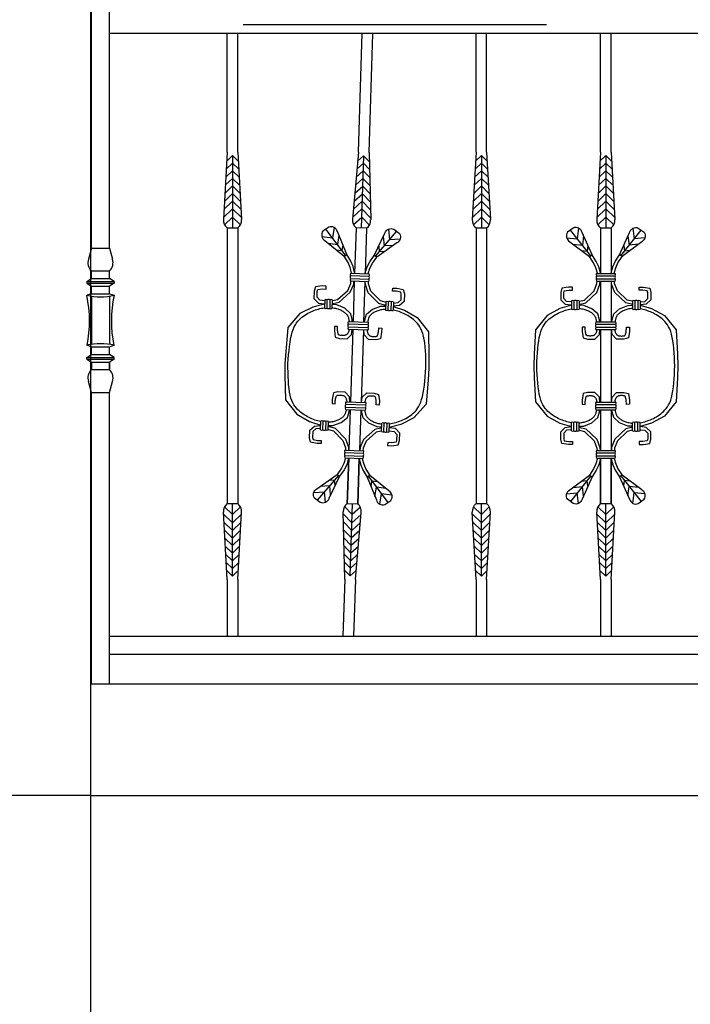
# Model space of a CAD drawing. Units: inches. Extents: x 2278 to 7495, y -71 to 1198.
# Tile 10 of 44: x 4871 to 4907, y 107 to 160. Entities that reach past the tile are written whole.
import ezdxf

# ---------------------------------------------------------------- set-up
doc = ezdxf.new("R2010")
doc.units = ezdxf.units.IN
doc.header["$MEASUREMENT"] = 0
doc.layers.add('A-ANNO-DIMS', color=2, linetype='Continuous', lineweight=18)
doc.layers.add('A-ELEV', color=7, linetype='Continuous', lineweight=25)
doc.styles.get("Standard").update_dxf_attribs({"font": 'arial.ttf'})
doc.dimstyles.get("Standard").update_dxf_attribs({"dimtxt": 6, "dimasz": 3, "dimexe": 0.18, "dimexo": 0.0625, "dimgap": 0.09, "dimtad": 0, "dimtih": 1, "dimtoh": 1, "dimdec": 0, "dimzin": 0, "dimdsep": 46, "dimlunit": 3, "dimtxsty": 'Standard', "dimblk": 'ARCHTICK', "dimcen": 0.09, "dimadec": 0, "dimazin": 0, "dimtfac": 1, "dimtdec": 0, "dimtofl": 0, "dimtmove": 0, "dimatfit": 3, "dimfxl": 1, "dimtolj": 1, "dimtzin": 0, "dimarcsym": 0})

# ---------------------------------------------------------------- blocks, each defined once
blk = doc.blocks.new('BALUSTER-ORNATE-C')
for p, q in [((3.585, 26.003), (3.585, 32.384)), ((4.155, 26.003), (4.155, 32.38)), ((3.585, 26.003), (3.383, 22.393)), ((4.155, 26.003), (4.357, 22.393)), ((3.533, 25.084), (3.87, 25.41)), ((3.557, 25.516), (3.87, 25.818)), ((3.87, 25.818), (3.87, 21.929)), ((4.182, 25.516), (3.87, 25.818)), ((4.206, 25.084), (3.87, 25.41)), ((3.509, 24.653), (3.87, 25.001)), ((4.231, 24.653), (3.87, 25.001)), ((3.485, 24.221), (3.87, 24.593)), ((4.255, 24.221), (3.87, 24.593)), ((3.461, 23.79), (3.87, 24.185)), ((4.279, 23.79), (3.87, 24.185)), ((3.412, 22.927), (3.87, 23.369)), ((3.437, 23.358), (3.87, 23.777)), ((4.303, 23.358), (3.87, 23.777)), ((4.327, 22.927), (3.87, 23.369)), ((3.388, 22.495), (3.87, 22.961)), ((4.351, 22.495), (3.87, 22.961)), ((3.441, 22.106), (3.87, 22.52)), ((4.298, 22.106), (3.87, 22.52)), ((3.063, 20.442), (1.97, 21.814)), ((2.412, 21.914), (2.338, 21.352)), ((3.585, 21.929), (3.585, 19.485)), ((4.155, 21.929), (3.585, 21.929)), ((4.155, 21.929), (4.155, 19.485)), ((4.677, 20.442), (5.769, 21.814)), ((5.328, 21.914), (5.401, 21.352)), ((1.774, 21.406), (2.338, 21.352)), ((2.678, 21.507), (2.613, 21.007)), ((5.061, 21.507), (5.127, 21.007)), ((5.966, 21.406), (5.401, 21.352)), ((2.111, 21.055), (2.613, 21.007)), ((2.562, 20.717), (2.867, 20.688)), ((2.907, 20.992), (2.867, 20.688)), ((4.833, 20.992), (4.872, 20.688)), ((5.177, 20.717), (4.872, 20.688)), ((5.629, 21.055), (5.127, 21.007)), ((3.37, 19.485), (4.37, 19.485)), ((3.37, 19.363), (4.37, 19.363)), ((3.37, 19.2), (4.37, 19.2)), ((3.37, 19.077), (4.37, 19.077)), ((3.585, 19.077), (3.585, 16.887)), ((4.155, 19.077), (4.155, 16.887)), ((2.026, 18.021), (2.026, 17.565)), ((2.148, 18.021), (2.148, 17.565)), ((2.311, 18.021), (2.311, 17.565)), ((2.433, 18.021), (2.433, 17.565)), ((5.306, 18.021), (5.306, 17.565)), ((5.428, 18.021), (5.428, 17.565)), ((5.591, 18.021), (5.591, 17.565)), ((5.714, 18.021), (5.714, 17.565)), ((3.329, 16.887), (4.411, 16.887)), ((3.329, 16.764), (4.411, 16.764)), ((3.329, 16.601), (4.411, 16.601)), ((3.329, 16.479), (4.411, 16.479)), ((3.585, 16.479), (3.585, 12.578)), ((4.155, 16.479), (4.155, 12.578)), ((3.329, 12.578), (4.411, 12.578)), ((3.329, 12.456), (4.411, 12.456)), ((3.329, 12.293), (4.411, 12.293)), ((3.329, 12.171), (4.411, 12.171)), ((3.585, 12.171), (3.585, 9.98)), ((4.155, 12.171), (4.155, 9.98)), ((2.026, 11.037), (2.026, 11.493)), ((2.148, 11.037), (2.148, 11.493)), ((2.311, 11.037), (2.311, 11.493)), ((2.433, 11.037), (2.433, 11.493)), ((5.306, 11.037), (5.306, 11.493)), ((5.428, 11.037), (5.428, 11.493)), ((5.591, 11.037), (5.591, 11.493)), ((5.714, 11.037), (5.714, 11.493)), ((3.37, 9.98), (4.37, 9.98)), ((3.37, 9.858), (4.37, 9.858)), ((3.37, 9.695), (4.37, 9.695)), ((3.37, 9.573), (4.37, 9.573)), ((3.585, 9.573), (3.585, 7.095)), ((3.585, 7.095), (3.585, 9.573)), ((4.155, 9.573), (4.155, 7.095)), ((4.155, 7.095), (4.155, 9.573)), ((3.063, 8.615), (1.97, 7.244)), ((4.677, 8.615), (5.769, 7.244)), ((2.111, 8.002), (2.613, 8.051)), ((2.562, 8.34), (2.867, 8.37)), ((2.678, 7.551), (2.613, 8.051)), ((2.907, 8.066), (2.867, 8.37)), ((4.833, 8.066), (4.872, 8.37)), ((5.177, 8.34), (4.872, 8.37)), ((5.061, 7.551), (5.127, 8.051)), ((5.629, 8.002), (5.127, 8.051)), ((1.774, 7.651), (2.338, 7.706)), ((2.412, 7.143), (2.338, 7.706)), ((5.328, 7.143), (5.401, 7.706)), ((5.966, 7.651), (5.401, 7.706)), ((3.441, 6.952), (3.87, 6.538)), ((3.585, 7.128), (4.155, 7.128)), ((3.87, 3.24), (3.87, 7.128)), ((4.298, 6.952), (3.87, 6.538)), ((3.585, 3.055), (3.383, 6.664)), ((3.388, 6.562), (3.87, 6.097)), ((4.351, 6.562), (3.87, 6.097)), ((4.155, 3.055), (4.357, 6.664)), ((3.412, 6.131), (3.87, 5.689)), ((4.327, 6.131), (3.87, 5.689)), ((3.437, 5.699), (3.87, 5.28)), ((4.303, 5.699), (3.87, 5.28)), ((3.461, 5.268), (3.87, 4.872)), ((3.485, 4.836), (3.87, 4.464)), ((4.279, 5.268), (3.87, 4.872)), ((4.255, 4.836), (3.87, 4.464)), ((3.509, 4.405), (3.87, 4.056)), ((4.231, 4.405), (3.87, 4.056)), ((3.533, 3.973), (3.87, 3.648)), ((4.206, 3.973), (3.87, 3.648)), ((3.557, 3.542), (3.87, 3.24)), ((4.182, 3.542), (3.87, 3.24)), ((3.585, 3.055), (3.585, 0)), ((4.155, 3.055), (4.155, 0))]:
    blk.add_line(p, q)
for points in [[(3.131, 20.487), (2.594, 21.696, 0.435351), (2.128, 21.929), (1.813, 21.699, 0.435351), (1.936, 21.192), (2.995, 20.398)], [(4.608, 20.487), (5.145, 21.696, -0.435351), (5.612, 21.929), (5.927, 21.699, -0.435351), (5.804, 21.192), (4.745, 20.398)], [(3.131, 8.571), (2.594, 7.362, -0.435351), (2.128, 7.128), (1.813, 7.359, -0.435351), (1.936, 7.866), (2.995, 8.66)], [(4.608, 8.571), (5.145, 7.362, 0.435351), (5.612, 7.128), (5.927, 7.359, 0.435351), (5.804, 7.866), (4.745, 8.66)]]:
    blk.add_lwpolyline(points, format="xyb", close=True)
for points in [[(3.42, 19.485), (3.421, 19.506), (3.336, 19.795), (3.216, 20.057), (2.995, 20.398)], [(3.583, 19.485), (3.585, 19.526), (3.489, 19.852), (3.359, 20.135), (3.131, 20.487)], [(4.157, 19.485), (4.155, 19.526), (4.25, 19.852), (4.38, 20.135), (4.608, 20.487)], [(4.32, 19.485), (4.319, 19.506), (4.403, 19.795), (4.523, 20.057), (4.745, 20.398)], [(2.433, 17.826), (2.492, 17.833), (2.801, 17.915), (3.385, 18.463), (3.557, 18.908), (3.565, 19.077)], [(2.433, 17.99), (2.462, 17.993), (2.719, 18.062), (3.247, 18.557), (3.396, 18.942), (3.402, 19.077)], [(5.306, 17.826), (5.247, 17.833), (4.939, 17.915), (4.355, 18.463), (4.182, 18.908), (4.175, 19.077)], [(5.306, 17.99), (5.278, 17.993), (5.02, 18.062), (4.493, 18.557), (4.344, 18.942), (4.338, 19.077)], [(2.026, 17.961), (1.767, 17.989), (1.612, 18.138), (1.612, 18.447), (1.642, 18.56), (1.879, 18.596), (2.084, 18.596), (2.084, 18.759), (1.866, 18.759), (1.512, 18.705), (1.449, 18.469), (1.449, 18.069), (1.694, 17.833), (2.026, 17.797)], [(5.714, 17.961), (5.973, 17.989), (6.128, 18.138), (6.128, 18.447), (6.098, 18.56), (5.861, 18.596), (5.656, 18.596), (5.656, 18.759), (5.873, 18.759), (6.227, 18.705), (6.291, 18.469), (6.291, 18.069), (6.046, 17.833), (5.714, 17.797)], [(2.026, 17.782), (1.412, 17.603), (0.722, 17.231), (0.095, 16.469), (0.025, 15.162), (0, 14.529), (0.025, 13.895), (0.095, 12.589), (0.722, 11.827), (1.412, 11.455), (2.026, 11.276)], [(0.163, 14.522), (0.173, 14.759), (0.184, 14.995), (0.199, 15.227), (0.217, 15.452), (0.239, 15.667), (0.267, 15.87), (0.3, 16.057), (0.34, 16.227), (0.386, 16.376), (0.438, 16.508), (0.495, 16.624), (0.557, 16.727), (0.623, 16.819), (0.692, 16.9), (0.764, 16.975), (0.839, 17.043), (0.916, 17.105), (0.993, 17.163), (1.071, 17.216), (1.15, 17.265), (1.229, 17.309), (1.309, 17.35), (1.389, 17.388), (1.469, 17.422), (1.548, 17.454), (1.627, 17.484), (1.705, 17.51), (1.782, 17.533), (1.858, 17.553), (1.933, 17.571), (2.007, 17.585), (2.026, 17.587)], [(3.541, 16.887), (3.527, 17.004), (3.446, 17.313), (3.128, 17.594), (2.683, 17.766), (2.433, 17.777)], [(2.433, 17.606), (2.499, 17.6), (2.563, 17.592), (2.624, 17.582), (2.683, 17.57), (2.739, 17.556), (2.792, 17.54), (2.842, 17.522), (2.891, 17.503), (2.937, 17.482), (2.981, 17.46), (3.023, 17.436), (3.064, 17.41), (3.102, 17.384), (3.138, 17.357), (3.171, 17.329), (3.201, 17.301), (3.228, 17.272), (3.251, 17.244), (3.271, 17.217), (3.288, 17.19), (3.303, 17.162), (3.316, 17.134), (3.327, 17.104), (3.337, 17.072), (3.345, 17.038), (3.354, 17.001), (3.361, 16.962), (3.368, 16.922), (3.374, 16.887)], [(4.198, 16.887), (4.212, 17.004), (4.294, 17.313), (4.612, 17.594), (5.057, 17.766), (5.306, 17.777)], [(5.306, 17.606), (5.241, 17.6), (5.177, 17.592), (5.115, 17.582), (5.057, 17.57), (5.001, 17.556), (4.948, 17.54), (4.897, 17.522), (4.849, 17.503), (4.803, 17.482), (4.759, 17.46), (4.716, 17.436), (4.676, 17.41), (4.638, 17.384), (4.602, 17.357), (4.569, 17.329), (4.539, 17.301), (4.512, 17.272), (4.488, 17.244), (4.468, 17.217), (4.451, 17.19), (4.437, 17.162), (4.424, 17.134), (4.413, 17.104), (4.403, 17.072), (4.394, 17.038), (4.386, 17.001), (4.379, 16.962), (4.371, 16.922), (4.366, 16.887)], [(5.714, 17.782), (6.328, 17.603), (7.018, 17.231), (7.644, 16.469), (7.715, 15.162), (7.74, 14.529), (7.715, 13.895), (7.644, 12.589), (7.018, 11.827), (6.328, 11.455), (5.714, 11.276)], [(7.577, 14.522), (7.567, 14.759), (7.555, 14.995), (7.541, 15.227), (7.523, 15.452), (7.501, 15.667), (7.473, 15.87), (7.44, 16.057), (7.4, 16.227), (7.354, 16.376), (7.302, 16.508), (7.244, 16.624), (7.183, 16.727), (7.117, 16.819), (7.048, 16.9), (6.976, 16.975), (6.901, 17.043), (6.824, 17.105), (6.747, 17.163), (6.668, 17.216), (6.59, 17.265), (6.51, 17.309), (6.431, 17.35), (6.351, 17.388), (6.271, 17.422), (6.191, 17.454), (6.113, 17.484), (6.035, 17.51), (5.958, 17.533), (5.882, 17.553), (5.807, 17.571), (5.733, 17.585), (5.714, 17.587)], [(3.388, 16.479), (3.383, 16.441), (3.376, 16.401), (3.368, 16.364), (3.357, 16.329), (3.346, 16.299), (3.333, 16.271), (3.318, 16.247), (3.303, 16.225), (3.286, 16.207), (3.268, 16.19), (3.249, 16.176), (3.228, 16.164), (3.205, 16.154), (3.179, 16.145), (3.149, 16.138), (3.116, 16.133), (3.081, 16.13), (3.045, 16.129), (3.007, 16.129), (2.971, 16.131), (2.936, 16.134), (2.905, 16.137), (2.88, 16.142), (2.863, 16.146), (2.852, 16.151), (2.845, 16.154), (2.84, 16.159), (2.834, 16.166), (2.825, 16.18), (2.814, 16.203), (2.803, 16.237), (2.792, 16.28), (2.783, 16.331), (2.775, 16.388), (2.769, 16.452), (2.766, 16.522), (2.764, 16.599), (2.601, 16.596), (2.601, 16.378), (2.656, 16.024), (2.892, 15.961), (3.291, 15.961), (3.527, 16.206), (3.557, 16.479)], [(4.352, 16.479), (4.357, 16.441), (4.364, 16.401), (4.372, 16.364), (4.382, 16.329), (4.394, 16.299), (4.407, 16.271), (4.421, 16.247), (4.437, 16.225), (4.454, 16.207), (4.472, 16.19), (4.491, 16.176), (4.512, 16.164), (4.534, 16.154), (4.56, 16.145), (4.59, 16.138), (4.623, 16.133), (4.659, 16.13), (4.695, 16.129), (4.732, 16.129), (4.769, 16.131), (4.804, 16.134), (4.835, 16.137), (4.86, 16.142), (4.877, 16.146), (4.888, 16.151), (4.894, 16.154), (4.899, 16.159), (4.906, 16.166), (4.914, 16.18), (4.925, 16.203), (4.937, 16.237), (4.948, 16.28), (4.957, 16.331), (4.965, 16.388), (4.971, 16.452), (4.974, 16.522), (4.975, 16.599), (5.138, 16.596), (5.138, 16.378), (5.084, 16.024), (4.848, 15.961), (4.448, 15.961), (4.212, 16.206), (4.182, 16.479)], [(2.026, 11.47), (2.007, 11.473), (1.933, 11.487), (1.858, 11.504), (1.782, 11.524), (1.705, 11.548), (1.627, 11.574), (1.548, 11.603), (1.469, 11.635), (1.389, 11.67), (1.309, 11.708), (1.229, 11.748), (1.15, 11.793), (1.071, 11.841), (0.993, 11.894), (0.916, 11.952), (0.839, 12.015), (0.764, 12.083), (0.692, 12.157), (0.623, 12.239), (0.557, 12.33), (0.495, 12.433), (0.438, 12.549), (0.386, 12.681), (0.34, 12.831), (0.3, 13), (0.267, 13.188), (0.239, 13.391), (0.217, 13.606), (0.199, 13.831), (0.184, 14.062), (0.173, 14.298), (0.163, 14.536)], [(5.714, 11.47), (5.733, 11.473), (5.807, 11.487), (5.882, 11.504), (5.958, 11.524), (6.035, 11.548), (6.113, 11.574), (6.191, 11.603), (6.271, 11.635), (6.351, 11.67), (6.431, 11.708), (6.51, 11.748), (6.59, 11.793), (6.668, 11.841), (6.747, 11.894), (6.824, 11.952), (6.901, 12.015), (6.976, 12.083), (7.048, 12.157), (7.117, 12.239), (7.183, 12.33), (7.244, 12.433), (7.302, 12.549), (7.354, 12.681), (7.4, 12.831), (7.44, 13), (7.473, 13.188), (7.501, 13.391), (7.523, 13.606), (7.541, 13.831), (7.555, 14.062), (7.567, 14.298), (7.577, 14.536)], [(3.557, 12.578), (3.527, 12.852), (3.291, 13.097), (2.892, 13.097), (2.656, 13.033), (2.601, 12.679), (2.601, 12.462), (2.764, 12.459), (2.766, 12.536), (2.769, 12.605), (2.775, 12.669), (2.783, 12.727), (2.792, 12.778), (2.803, 12.82), (2.814, 12.854), (2.825, 12.878), (2.834, 12.892), (2.84, 12.899), (2.845, 12.903), (2.852, 12.907), (2.863, 12.911), (2.88, 12.916), (2.905, 12.92), (2.936, 12.924), (2.971, 12.927), (3.007, 12.929), (3.045, 12.929), (3.081, 12.928), (3.116, 12.924), (3.149, 12.919), (3.179, 12.912), (3.205, 12.904), (3.228, 12.893), (3.249, 12.881), (3.268, 12.867), (3.286, 12.851), (3.303, 12.832), (3.318, 12.811), (3.333, 12.786), (3.346, 12.759), (3.357, 12.728), (3.368, 12.694), (3.376, 12.656), (3.383, 12.616), (3.388, 12.578)], [(4.182, 12.578), (4.212, 12.852), (4.448, 13.097), (4.848, 13.097), (5.084, 13.033), (5.138, 12.679), (5.138, 12.462), (4.975, 12.459), (4.974, 12.536), (4.971, 12.605), (4.965, 12.669), (4.957, 12.727), (4.948, 12.778), (4.937, 12.82), (4.925, 12.854), (4.914, 12.878), (4.906, 12.892), (4.899, 12.899), (4.894, 12.903), (4.888, 12.907), (4.877, 12.911), (4.86, 12.916), (4.835, 12.92), (4.804, 12.924), (4.769, 12.927), (4.732, 12.929), (4.695, 12.929), (4.659, 12.928), (4.623, 12.924), (4.59, 12.919), (4.56, 12.912), (4.534, 12.904), (4.512, 12.893), (4.491, 12.881), (4.472, 12.867), (4.454, 12.851), (4.437, 12.832), (4.421, 12.811), (4.407, 12.786), (4.394, 12.759), (4.382, 12.728), (4.372, 12.694), (4.364, 12.656), (4.357, 12.616), (4.352, 12.578)], [(3.374, 12.171), (3.368, 12.136), (3.361, 12.095), (3.354, 12.056), (3.345, 12.02), (3.337, 11.986), (3.327, 11.954), (3.316, 11.924), (3.303, 11.895), (3.288, 11.868), (3.271, 11.841), (3.251, 11.813), (3.228, 11.785), (3.201, 11.757), (3.171, 11.729), (3.138, 11.701), (3.102, 11.673), (3.064, 11.647), (3.023, 11.622), (2.981, 11.598), (2.937, 11.576), (2.891, 11.555), (2.842, 11.535), (2.792, 11.518), (2.739, 11.502), (2.683, 11.488), (2.624, 11.476), (2.563, 11.465), (2.499, 11.457), (2.433, 11.451)], [(2.433, 11.28), (2.683, 11.291), (3.128, 11.464), (3.446, 11.745), (3.527, 12.053), (3.541, 12.171)], [(5.306, 11.28), (5.057, 11.291), (4.612, 11.464), (4.294, 11.745), (4.212, 12.053), (4.198, 12.171)], [(4.366, 12.171), (4.371, 12.136), (4.379, 12.095), (4.386, 12.056), (4.394, 12.02), (4.403, 11.986), (4.413, 11.954), (4.424, 11.924), (4.437, 11.895), (4.451, 11.868), (4.468, 11.841), (4.488, 11.813), (4.512, 11.785), (4.539, 11.757), (4.569, 11.729), (4.602, 11.701), (4.638, 11.673), (4.676, 11.647), (4.716, 11.622), (4.759, 11.598), (4.803, 11.576), (4.849, 11.555), (4.897, 11.535), (4.948, 11.518), (5.001, 11.502), (5.057, 11.488), (5.115, 11.476), (5.177, 11.465), (5.241, 11.457), (5.306, 11.451)], [(2.026, 11.097), (1.767, 11.069), (1.612, 10.919), (1.612, 10.611), (1.642, 10.498), (1.879, 10.461), (2.084, 10.461), (2.084, 10.298), (1.866, 10.298), (1.512, 10.353), (1.449, 10.589), (1.449, 10.988), (1.694, 11.225), (2.026, 11.261)], [(2.433, 11.232), (2.492, 11.225), (2.801, 11.143), (3.385, 10.594), (3.557, 10.149), (3.565, 9.98)], [(5.306, 11.232), (5.247, 11.225), (4.939, 11.143), (4.355, 10.594), (4.182, 10.149), (4.175, 9.98)], [(5.714, 11.097), (5.973, 11.069), (6.128, 10.919), (6.128, 10.611), (6.098, 10.498), (5.861, 10.461), (5.656, 10.461), (5.656, 10.298), (5.873, 10.298), (6.227, 10.353), (6.291, 10.589), (6.291, 10.988), (6.046, 11.225), (5.714, 11.261)], [(2.433, 11.067), (2.462, 11.064), (2.719, 10.996), (3.247, 10.501), (3.396, 10.115), (3.402, 9.98)], [(5.306, 11.067), (5.278, 11.064), (5.02, 10.996), (4.493, 10.501), (4.344, 10.115), (4.338, 9.98)], [(3.42, 9.573), (3.421, 9.552), (3.336, 9.262), (3.216, 9.001), (2.995, 8.66)], [(3.583, 9.573), (3.585, 9.532), (3.489, 9.205), (3.359, 8.922), (3.131, 8.571)], [(4.157, 9.573), (4.155, 9.532), (4.25, 9.205), (4.38, 8.922), (4.608, 8.571)], [(4.32, 9.573), (4.319, 9.552), (4.403, 9.262), (4.523, 9.001), (4.745, 8.66)]]:
    blk.add_lwpolyline(points)
for centre, radius, start, end in [((3.929, 22.355), 0.547, 176.0178, 231.0717), ((3.811, 22.355), 0.547, 308.9283, 3.9822), ((3.475, 19.424), 0.121, 149.7768, 210.2232), ((3.563, 19.281), 0.209, 157.1017, 202.8983), ((3.475, 19.139), 0.121, 149.7768, 210.2232), ((4.265, 19.424), 0.121, 329.7768, 30.2232), ((4.177, 19.281), 0.209, 337.1017, 22.8983), ((4.265, 19.139), 0.121, 329.7768, 30.2232), ((2.087, 17.916), 0.121, 59.7768, 120.2232), ((2.23, 17.828), 0.209, 67.1017, 112.8983), ((2.372, 17.916), 0.121, 59.7768, 120.2232), ((5.367, 17.916), 0.121, 59.7768, 120.2232), ((5.51, 17.828), 0.209, 67.1017, 112.8983), ((5.653, 17.916), 0.121, 59.7768, 120.2232), ((2.087, 17.67), 0.121, 239.7768, 300.2232), ((2.23, 17.758), 0.209, 247.1017, 292.8983), ((2.372, 17.67), 0.121, 239.7768, 300.2232), ((5.367, 17.67), 0.121, 239.7768, 300.2232), ((5.51, 17.758), 0.209, 247.1017, 292.8983), ((5.653, 17.67), 0.121, 239.7768, 300.2232), ((3.434, 16.825), 0.121, 149.7768, 210.2232), ((3.522, 16.683), 0.209, 157.1017, 202.8983), ((3.434, 16.54), 0.121, 149.7768, 210.2232), ((4.306, 16.825), 0.121, 329.7768, 30.2232), ((4.218, 16.683), 0.209, 337.1017, 22.8983), ((4.306, 16.54), 0.121, 329.7768, 30.2232), ((3.434, 12.517), 0.121, 149.7768, 210.2232), ((3.522, 12.375), 0.209, 157.1017, 202.8983), ((3.434, 12.232), 0.121, 149.7768, 210.2232), ((4.306, 12.517), 0.121, 329.7768, 30.2232), ((4.218, 12.375), 0.209, 337.1017, 22.8983), ((4.306, 12.232), 0.121, 329.7768, 30.2232), ((2.087, 11.388), 0.121, 59.7768, 120.2232), ((2.23, 11.3), 0.209, 67.1017, 112.8983), ((2.372, 11.388), 0.121, 59.7768, 120.2232), ((5.367, 11.388), 0.121, 59.7768, 120.2232), ((5.51, 11.3), 0.209, 67.1017, 112.8983), ((5.653, 11.388), 0.121, 59.7768, 120.2232), ((2.087, 11.142), 0.121, 239.7768, 300.2232), ((2.23, 11.23), 0.209, 247.1017, 292.8983), ((2.372, 11.142), 0.121, 239.7768, 300.2232), ((5.367, 11.142), 0.121, 239.7768, 300.2232), ((5.51, 11.23), 0.209, 247.1017, 292.8983), ((5.653, 11.142), 0.121, 239.7768, 300.2232), ((3.475, 9.919), 0.121, 149.7768, 210.2232), ((3.563, 9.776), 0.209, 157.1017, 202.8983), ((3.475, 9.634), 0.121, 149.7768, 210.2232), ((4.265, 9.919), 0.121, 329.7768, 30.2232), ((4.177, 9.776), 0.209, 337.1017, 22.8983), ((4.265, 9.634), 0.121, 329.7768, 30.2232), ((3.929, 6.703), 0.547, 128.9283, 183.9822), ((3.811, 6.703), 0.547, 356.0178, 51.0717)]:
    blk.add_arc(centre, radius, start, end)
blk = doc.blocks.new('RAIL-BAR-A')
for p, q in [((0.202, 26.003), (0.202, 32.38)), ((0.773, 26.003), (0.773, 32.38)), ((0.202, 26.003), (0, 22.393)), ((0.773, 26.003), (0.975, 22.393)), ((0.151, 25.084), (0.488, 25.41)), ((0.175, 25.516), (0.488, 25.818)), ((0.488, 25.818), (0.488, 21.929)), ((0.8, 25.516), (0.488, 25.818)), ((0.824, 25.084), (0.488, 25.41)), ((0.127, 24.653), (0.488, 25.001)), ((0.848, 24.653), (0.488, 25.001)), ((0.103, 24.221), (0.488, 24.593)), ((0.873, 24.221), (0.488, 24.593)), ((0.079, 23.79), (0.488, 24.185)), ((0.897, 23.79), (0.488, 24.185)), ((0.03, 22.927), (0.488, 23.369)), ((0.054, 23.358), (0.488, 23.777)), ((0.921, 23.358), (0.488, 23.777)), ((0.945, 22.927), (0.488, 23.369)), ((0.006, 22.495), (0.488, 22.961)), ((0.969, 22.495), (0.488, 22.961)), ((0.059, 22.106), (0.488, 22.52)), ((0.916, 22.106), (0.488, 22.52)), ((0.202, 21.929), (0.202, 7.128)), ((0.773, 21.929), (0.202, 21.929)), ((0.773, 21.929), (0.773, 7.128)), ((0.059, 6.952), (0.488, 6.538)), ((0.202, 7.128), (0.773, 7.128)), ((0.488, 3.24), (0.488, 7.128)), ((0.916, 6.952), (0.488, 6.538)), ((0.202, 3.055), (0, 6.664)), ((0.006, 6.562), (0.488, 6.097)), ((0.969, 6.562), (0.488, 6.097)), ((0.773, 3.055), (0.975, 6.664)), ((0.03, 6.131), (0.488, 5.689)), ((0.945, 6.131), (0.488, 5.689)), ((0.054, 5.699), (0.488, 5.28)), ((0.921, 5.699), (0.488, 5.28)), ((0.079, 5.268), (0.488, 4.872)), ((0.103, 4.836), (0.488, 4.464)), ((0.897, 5.268), (0.488, 4.872)), ((0.873, 4.836), (0.488, 4.464)), ((0.127, 4.405), (0.488, 4.056)), ((0.848, 4.405), (0.488, 4.056)), ((0.151, 3.973), (0.488, 3.648)), ((0.824, 3.973), (0.488, 3.648)), ((0.175, 3.542), (0.488, 3.24)), ((0.8, 3.542), (0.488, 3.24)), ((0.202, 3.055), (0.202, 0)), ((0.773, 3.055), (0.773, 0))]:
    blk.add_line(p, q)
for centre, start, end in [((0.546, 22.355), 176.0178, 231.0717), ((0.429, 22.355), 308.9283, 3.9822), ((0.546, 6.703), 128.9283, 183.9822), ((0.429, 6.703), 356.0178, 51.0717)]:
    blk.add_arc(centre, 0.547, start, end)
blk = doc.blocks.new('RAIL-BAR-B')
for p, q in [((17.353, 32.832), (1.059, 32.832)), ((0.203, 26.003), (0.203, 32.38)), ((0.773, 26.003), (0.773, 32.38)), ((0.203, 26.003), (0.001, 22.393)), ((0.773, 26.003), (0.976, 22.393)), ((0.152, 25.084), (0.488, 25.41)), ((0.176, 25.516), (0.488, 25.818)), ((0.488, 25.818), (0.488, 21.929)), ((0.801, 25.516), (0.488, 25.818)), ((0.825, 25.084), (0.488, 25.41)), ((0.128, 24.653), (0.488, 25.001)), ((0.849, 24.653), (0.488, 25.001)), ((0.103, 24.221), (0.488, 24.593)), ((0.873, 24.221), (0.488, 24.593)), ((0.079, 23.79), (0.488, 24.185)), ((0.897, 23.79), (0.488, 24.185)), ((0.031, 22.927), (0.488, 23.369)), ((0.055, 23.358), (0.488, 23.777)), ((0.922, 23.358), (0.488, 23.777)), ((0.946, 22.927), (0.488, 23.369)), ((0.007, 22.495), (0.488, 22.961)), ((0.97, 22.495), (0.488, 22.961)), ((0.06, 22.106), (0.488, 22.52)), ((0.917, 22.106), (0.488, 22.52)), ((0.203, 21.929), (0.203, 7.128)), ((0.773, 21.929), (0.203, 21.929)), ((0.773, 21.929), (0.773, 7.128)), ((0.06, 6.952), (0.488, 6.538)), ((0.203, 7.128), (0.773, 7.128)), ((0.488, 3.24), (0.488, 7.128)), ((0.917, 6.952), (0.488, 6.538)), ((0.203, 3.055), (0.001, 6.664)), ((0.007, 6.562), (0.488, 6.097)), ((0.97, 6.562), (0.488, 6.097)), ((0.773, 3.055), (0.976, 6.664)), ((0.031, 6.131), (0.488, 5.689)), ((0.946, 6.131), (0.488, 5.689)), ((0.055, 5.699), (0.488, 5.28)), ((0.922, 5.699), (0.488, 5.28)), ((0.079, 5.268), (0.488, 4.872)), ((0.103, 4.836), (0.488, 4.464)), ((0.897, 5.268), (0.488, 4.872)), ((0.873, 4.836), (0.488, 4.464)), ((0.128, 4.405), (0.488, 4.056)), ((0.849, 4.405), (0.488, 4.056)), ((0.152, 3.973), (0.488, 3.648)), ((0.825, 3.973), (0.488, 3.648)), ((0.176, 3.542), (0.488, 3.24)), ((0.801, 3.542), (0.488, 3.24)), ((0.203, 3.055), (0.203, 0)), ((0.773, 3.055), (0.773, 0))]:
    blk.add_line(p, q)
for centre, start, end in [((0.547, 22.355), 176.0178, 231.0717), ((0.429, 22.355), 308.9283, 3.9822), ((0.547, 6.703), 128.9283, 183.9822), ((0.429, 6.703), 356.0178, 51.0717)]:
    blk.add_arc(centre, 0.547, start, end)
blk = doc.blocks.new('_ArchTick')
at = {"color": 0, "linetype": 'ByBlock', "const_width": 0.15}
blk.add_lwpolyline([(-0.5, -0.5), (0.5, 0.5)], dxfattribs=at)
blk = doc.blocks.new('*D123')
at = {"layer": 'A-ANNO-DIMS', "color": 0, "lineweight": -2, "transparency": 16777216}
for p, q in [((4736.95, 340.157), (4736.95, -23.427)), ((5145.676, -1.81), (5145.676, -23.427)), ((4736.95, -23.247), (4923.929, -23.247)), ((5145.676, -23.247), (4958.697, -23.247))]:
    blk.add_line(p, q, dxfattribs=at)
at = {"layer": 'Defpoints', "color": 0, "transparency": 16777216}
for p in [(4736.95, 340.219), (5145.676, -1.747), (5145.676, -23.247)]:
    blk.add_point(p, dxfattribs=at)
at = {"layer": 'A-ANNO-DIMS', "color": 0, "lineweight": -2, "transparency": 16777216, "xscale": 3, "yscale": 3, "zscale": 3, "rotation": 180}
blk.add_blockref('_ArchTick', (4736.95, -23.247), dxfattribs=at)
at = {"layer": 'A-ANNO-DIMS', "color": 0, "lineweight": -2, "transparency": 16777216, "xscale": 3, "yscale": 3, "zscale": 3}
blk.add_blockref('_ArchTick', (5145.676, -23.247), dxfattribs=at)
at = {"layer": 'A-ANNO-DIMS', "color": 0, "transparency": 16777216, "insert": (4941.313, -23.247), "char_height": 6, "attachment_point": 5}
blk.add_mtext('\\A1;34\'-0 1/2"', dxfattribs=at)
blk = doc.blocks.new('*D126')
at = {"layer": 'A-ANNO-DIMS', "color": 0, "lineweight": -2, "transparency": 16777216}
for p, q in [((4837.736, 313.27), (4837.736, 361.899)), ((4837.736, 361.719), (4848.143, 361.719)), ((4874.676, 361.719), (4864.269, 361.719)), ((4874.676, 99.315), (4874.676, 361.899))]:
    blk.add_line(p, q, dxfattribs=at)
at = {"layer": 'Defpoints', "color": 0, "transparency": 16777216}
for p in [(4874.676, 361.719), (4837.736, 313.208), (4874.676, 99.253)]:
    blk.add_point(p, dxfattribs=at)
at = {"layer": 'A-ANNO-DIMS', "color": 0, "lineweight": -2, "transparency": 16777216, "xscale": 3, "yscale": 3, "zscale": 3, "rotation": 180}
blk.add_blockref('_ArchTick', (4837.736, 361.719), dxfattribs=at)
at = {"layer": 'A-ANNO-DIMS', "color": 0, "lineweight": -2, "transparency": 16777216, "xscale": 3, "yscale": 3, "zscale": 3}
blk.add_blockref('_ArchTick', (4874.676, 361.719), dxfattribs=at)
at = {"layer": 'A-ANNO-DIMS', "color": 0, "transparency": 16777216, "insert": (4856.206, 361.719), "char_height": 6, "attachment_point": 5}
blk.add_mtext('\\A1;3\'-1"', dxfattribs=at)
blk = doc.blocks.new('*D127')
at = {"layer": 'A-ANNO-DIMS', "color": 0, "lineweight": -2, "transparency": 16777216}
for p, q in [((4874.676, 99.315), (4874.676, 361.899)), ((4874.676, 361.719), (4881.729, 361.719)), ((4909.676, 361.719), (4902.623, 361.719)), ((4909.676, 99.315), (4909.676, 361.899))]:
    blk.add_line(p, q, dxfattribs=at)
at = {"layer": 'Defpoints', "color": 0, "transparency": 16777216}
for p in [(4909.676, 361.719), (4874.676, 99.253), (4909.676, 99.253)]:
    blk.add_point(p, dxfattribs=at)
at = {"layer": 'A-ANNO-DIMS', "color": 0, "lineweight": -2, "transparency": 16777216, "xscale": 3, "yscale": 3, "zscale": 3, "rotation": 180}
blk.add_blockref('_ArchTick', (4874.676, 361.719), dxfattribs=at)
at = {"layer": 'A-ANNO-DIMS', "color": 0, "lineweight": -2, "transparency": 16777216, "xscale": 3, "yscale": 3, "zscale": 3}
blk.add_blockref('_ArchTick', (4909.676, 361.719), dxfattribs=at)
at = {"layer": 'A-ANNO-DIMS', "color": 0, "transparency": 16777216, "insert": (4892.176, 361.719), "char_height": 6, "attachment_point": 5}
blk.add_mtext('\\A1;2\'-11"', dxfattribs=at)

msp = doc.modelspace()

# ---------------------------------------------------------------- linework, layer by layer
at = {"layer": 'A-ELEV'}
for p, q in [((4874.676, 124.253), (4874.676, 250.253)), ((4874.696, 147.642), (4874.696, 161.577)), ((4875.673, 147.642), (4875.673, 161.577)), ((4969.039, 159.179), (4875.673, 159.179)), ((4874.696, 147.642), (4874.543, 147.049)), ((4874.696, 147.642), (4875.673, 147.642)), ((4875.673, 147.642), (4875.826, 147.049)), ((4874.451, 145.849), (4874.696, 146.012)), ((4874.696, 146.42), (4875.673, 146.42)), ((4874.696, 146.012), (4874.696, 146.42)), ((4874.696, 146.012), (4875.673, 146.012)), ((4875.673, 146.012), (4875.673, 146.42)), ((4875.918, 145.849), (4875.673, 146.012)), ((4874.451, 145.849), (4875.918, 145.849)), ((4874.451, 145.849), (4874.451, 145.768)), ((4874.451, 145.768), (4875.918, 145.768)), ((4874.451, 145.768), (4874.696, 145.605)), ((4874.696, 145.198), (4874.696, 145.605)), ((4874.696, 145.605), (4875.673, 145.605)), ((4875.918, 145.768), (4875.673, 145.605)), ((4875.673, 145.198), (4875.673, 145.605)), ((4875.918, 145.849), (4875.918, 145.768)), ((4874.696, 145.198), (4874.451, 145.116)), ((4874.696, 145.198), (4875.673, 145.198)), ((4874.696, 145.07), (4874.696, 142.474)), ((4875.673, 145.198), (4875.918, 145.116)), ((4875.673, 145.07), (4875.673, 142.474)), ((4874.696, 142.346), (4874.451, 142.428)), ((4874.696, 142.346), (4875.673, 142.346)), ((4874.696, 141.936), (4874.696, 142.346)), ((4875.673, 142.346), (4875.918, 142.428)), ((4875.673, 141.936), (4875.673, 142.346)), ((4874.451, 141.773), (4874.696, 141.936)), ((4874.451, 141.773), (4875.918, 141.773)), ((4874.451, 141.691), (4874.451, 141.773)), ((4874.696, 141.936), (4875.673, 141.936)), ((4875.918, 141.773), (4875.673, 141.936)), ((4875.918, 141.691), (4875.918, 141.773)), ((4874.451, 141.691), (4875.918, 141.691)), ((4874.451, 141.691), (4874.696, 141.529)), ((4874.696, 141.529), (4875.673, 141.529)), ((4874.696, 141.121), (4874.696, 141.529)), ((4874.696, 141.529), (4874.696, 141.121)), ((4875.918, 141.691), (4875.673, 141.529)), ((4875.673, 141.121), (4875.673, 141.529)), ((4875.673, 141.529), (4875.673, 141.121)), ((4874.696, 141.121), (4875.673, 141.121)), ((4874.696, 139.899), (4874.543, 140.492)), ((4875.673, 139.899), (4875.826, 140.492)), ((4874.696, 124.253), (4874.696, 139.899)), ((4874.696, 139.899), (4875.673, 139.899)), ((4875.673, 124.253), (4875.673, 139.899)), ((4969.039, 126.799), (4875.673, 126.799)), ((4969.039, 125.821), (4875.673, 125.821)), ((4874.676, 124.253), (5145.676, 124.253)), ((4874.676, 118.253), (4868.679, 118.253)), ((4874.676, 118.253), (5145.676, 118.253)), ((4874.676, 67.611), (4874.676, 118.253))]:
    msp.add_line(p, q, dxfattribs=at)
for centre, radius, start, end in [((4875.119, 146.856), 0.608, 161.4732, 225.8681), ((4875.25, 146.856), 0.608, 314.1319, 18.5268), ((4868.081, 143.743), 6.517, 348.3176, 12.1601), ((4875.185, 148.339), 3.305, 257.1818, 282.8182), ((4882.288, 143.743), 6.517, 167.8399, 191.6824), ((4875.185, 139.205), 3.305, 77.1818, 102.8182), ((4875.119, 140.685), 0.608, 134.1319, 198.5268), ((4875.25, 140.685), 0.608, 341.4732, 45.8681)]:
    msp.add_arc(centre, radius, start, end, dxfattribs=at)

# ---------------------------------------------------------------- block references
for name, p in [('RAIL-BAR-B', (4881.784, 126.799)), ('RAIL-BAR-A', (4895.146, 126.799)), ('BALUSTER-ORNATE-C', (4898.444, 126.799))]:
    msp.add_blockref(name, p, dxfattribs=at)
at = {"layer": 'A-ELEV', "rotation": 358.1715281196677}
msp.add_blockref('BALUSTER-ORNATE-C', (4884.622, 126.93), dxfattribs=at)

# ---------------------------------------------------------------- dimensions: what is measured, and where the dimension line sits
at = {"layer": 'A-ANNO-DIMS'}
for base, p1, p2, picture, middle in [((4874.676, 361.719), (4837.736, 313.208), (4874.676, 99.253), '*D126', (4856.206, 361.719)), ((4909.676, 361.719), (4874.676, 99.253), (4909.676, 99.253), '*D127', (4892.176, 361.719)), ((5145.676, -23.247), (4736.95, 340.219), (5145.676, -1.747), '*D123', (4941.313, -23.247))]:
    dim = msp.add_linear_dim(base=base, p1=p1, p2=p2, dimstyle='Standard', override={"dimdec": 1, "dimlfac": 1, "dimrnd": 0, "dimzin": 1, "dimdsep": 46, "dimlunit": 4, "dimfrac": 2}, dxfattribs=at)
    dim.commit()
    dim.dimension.update_dxf_attribs({"geometry": picture, "text_midpoint": middle})

doc.saveas('drawing.dxf')
